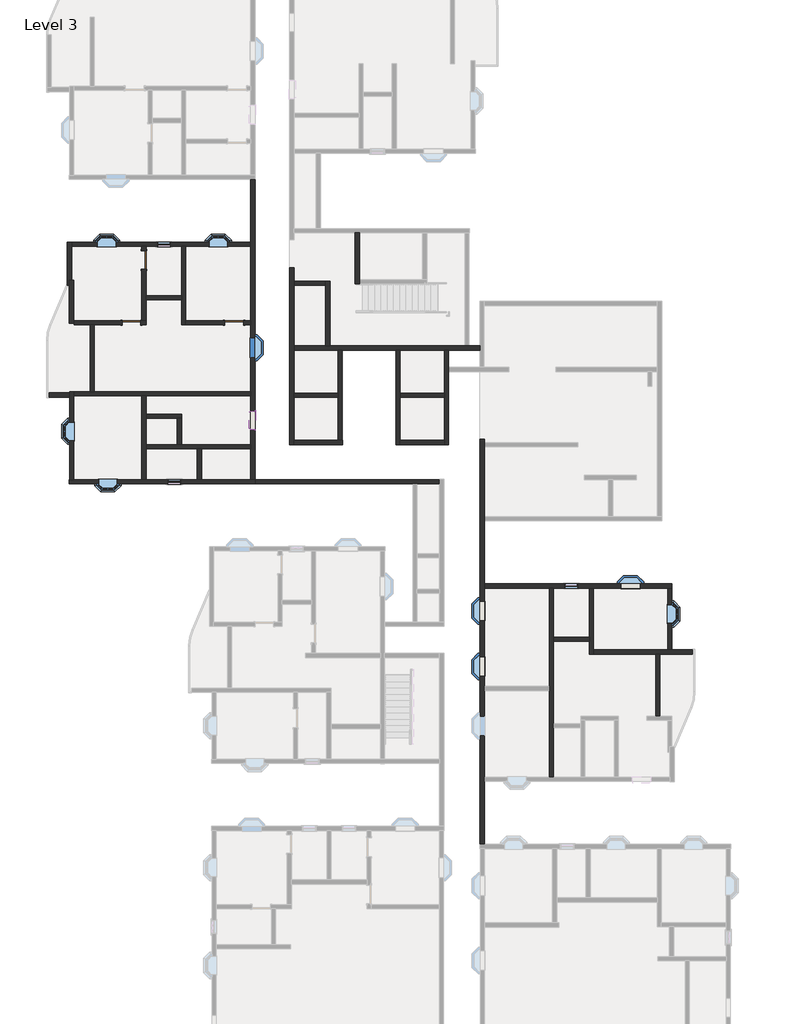
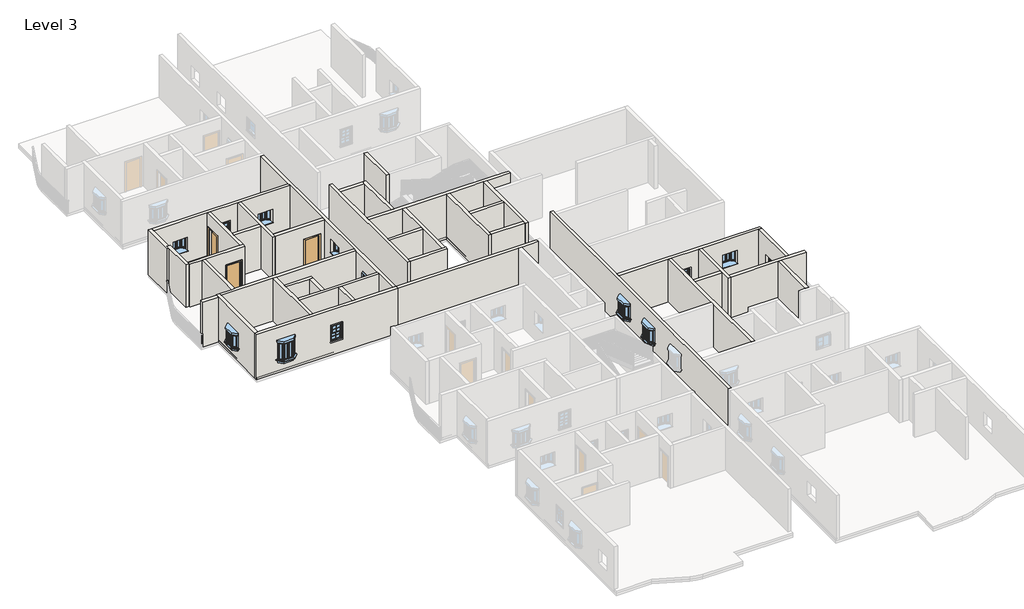
# One storey, part 3 of 14: 40 walls, 13 windows, 3 doors.
# Revit data of these elements (continued)
# Element 26 (IfcWall, "9\"")
#   Top Offset = 0' - 0"
#   Base Offset = 0' - 0"
#   wall height = 10' - 0"
#   Phase Created = New Construction
#   Base Constraint = Level 3
#   Top Constraint = Level 4
#   Materials on its faces: "Default Wall", "Earth"
# Element 27 (IfcWall, "9\"")
#   Top Offset = 0' - 0"
#   Base Offset = 0' - 0"
#   wall height = 10' - 0"
#   Phase Created = New Construction
#   Base Constraint = Level 3
#   Top Constraint = Level 4
#   Materials on its faces: "Default Wall", "Default Mass Interior Wall"
# Element 28 (IfcWall, "9\"")
#   Top Offset = 0' - 0"
#   Base Offset = 0' - 0"
#   wall height = 10' - 0"
#   Phase Created = New Construction
#   Base Constraint = Level 3
#   Top Constraint = Level 4
#   Materials on its faces: "Default Wall"
# Element 29 (IfcWall, "9\"")
#   Top Offset = 0' - 0"
#   Base Offset = 0' - 0"
#   wall height = 10' - 0"
#   Phase Created = New Construction
#   Base Constraint = Level 3
#   Top Constraint = Level 4
#   Materials on its faces: "Default Wall", "Default Mass Interior Wall", "Earth"
# Elements 30, 33, 34, 35, 36, 37, 38, 39, 40, 41 (IfcWall, "9\" w")
#   Top Offset = 0' - 0"
#   Base Offset = 0' - 0"
#   wall height = 10' - 0"
#   Phase Created = New Construction
#   Base Constraint = Level 3
#   Top Constraint = Level 4
#   Materials on its faces: "Default Wall"
# Element 31 (IfcWall, "9\" w")
#   Top Offset = 0' - 0"
#   Base Offset = 0' - 0"
#   wall height = 10' - 0"
#   Phase Created = New Construction
#   Base Constraint = Level 3
#   Top Constraint = Level 4
#   Materials on its faces: "Default Wall", "Earth"
# Element 32 (IfcWall, "9\" w")
#   Top Offset = 0' - 0"
#   Base Offset = 0' - 0"
#   wall height = 10' - 0"
#   Phase Created = New Construction
#   Base Constraint = Level 3
#   Top Constraint = Level 4
#   Materials on its faces: "Default Wall", "Brick, Soldier Course"
# Element 42 (IfcWall, "9\" w")
#   Top Offset = 0' - 0"
#   Base Offset = 0' - 0"
#   wall height = 10' - 0"
#   Phase Created = New Construction
#   Base Constraint = Level 3
#   Top Constraint = Level 4
#   Materials on its faces: "Default Wall", "Wood - Stained"
# Element 43 (IfcWall, "9\" w")
#   Top Offset = 0' - 0"
#   Base Offset = 0' - 0"
#   wall height = 10' - 0"
#   Phase Created = New Construction
#   Base Constraint = Level 3
#   Top Constraint = Level 4
#   Materials on its faces: "Default Wall", "Acoustic Ceiling Tile 24 x 24"
# Element 44 (IfcWindow, "910x1210mm")
#   Mark = "304"
#   Phase Created = New Construction
#   Materials on its faces: "Window Frame", "Glass"
# Element 45 (IfcWindow, "910x910mm")
#   Mark = "145"
#   Phase Created = New Construction
#   Materials on its faces: "Window Frame", "Glass"
# Element 46 (IfcWindow, "910x910mm")
#   Mark = "146"
#   Phase Created = New Construction
#   Materials on its faces: "Window Frame", "Glass"
# Element 47 (IfcWindow, "910x910mm")
#   Mark = "118"
#   Phase Created = New Construction
#   Materials on its faces: "Window Frame", "Glass"
# Element 48 (IfcWindow, "910x910mm")
#   Mark = "119"
#   Phase Created = New Construction
#   Materials on its faces: "Window Frame", "Glass"
# Element 49 (IfcWindow, "910x910mm")
#   Mark = "120"
#   Phase Created = New Construction
#   Materials on its faces: "Window Frame", "Glass"
# Element 50 (IfcWindow, "910x910mm")
#   Mark = "121"
#   Phase Created = New Construction
#   Materials on its faces: "Window Frame", "Glass"
# Element 51 (IfcWindow, "910x910mm")
#   Mark = "143"
#   Phase Created = New Construction
#   Materials on its faces: "Window Frame", "Glass"
# Element 52 (IfcWindow, "910x910mm")
#   Mark = "144"
#   Phase Created = New Construction
#   Materials on its faces: "Window Frame", "Glass"
# Element 53 (IfcWindow, "Window-Double-Hung : 26\" x 42\"")
#   Mark = "167"
#   Window Inset = 0' - 0"
#   Interior Wall Closure = 0' - 1 1/2"
#   Frame Extension = 0' - 1 1/4"
#   Exterior Wall Closure = 0' - 0 1/2"
#   Interior Trim Visibility = yes
#   Indicator Visibility = yes
#   Exterior Trim Visibility = yes
#   Phase Created = New Construction
#   Materials on its faces: "Wood - Stained", "Glass", "Clad - White"
# Element 54 (IfcWindow, "Window-Double-Hung : 26\" x 42\"")
#   Mark = "156"
#   Window Inset = 0' - 0"
#   Interior Wall Closure = 0' - 1 1/2"
#   Frame Extension = 0' - 1 1/4"
#   Exterior Wall Closure = 0' - 0 1/2"
#   Interior Trim Visibility = yes
#   Indicator Visibility = yes
#   Exterior Trim Visibility = yes
#   Phase Created = New Construction
#   Materials on its faces: "Wood - Stained", "Glass", "Clad - White"
# Element 55 (IfcWindow, "Window-Double-Hung : 26\" x 42\"")
#   Mark = "157"
#   Window Inset = 0' - 0"
#   Interior Wall Closure = 0' - 1 1/2"
#   Frame Extension = 0' - 1 1/4"
#   Exterior Wall Closure = 0' - 0 1/2"
#   Interior Trim Visibility = yes
#   Indicator Visibility = yes
#   Exterior Trim Visibility = yes
#   Phase Created = New Construction
#   Materials on its faces: "Wood - Stained", "Glass", "Clad - White"
# Element 56 (IfcWindow, "Windows_Sgl_w-Glazing_Bars : 910x910mm")
#   Mark = "152"
#   Phase Created = New Construction
#   Materials on its faces: "Window Frame", "Glass"
# Materials
#   "Door - Panel": class "Wood", colour RGB 210 159 95, transparency 0, Cost = 0
#   "Door - Frame": colour RGB 118 70 51, transparency 0, Cost = 0
#   "Window Frame": colour RGB 249 249 249, transparency 0
#   "Glass": class "Glass", colour RGB 0 128 192, transparency 0.75, Description = "Soda Lime Glass", Cost = 0
#   "Wood - Stained": class "Wood", colour RGB 224 178 126, transparency 0, Cost = 0
#   "Clad - White": class "Wood", colour RGB 242 242 238, transparency 0, Cost = 0
#   "Default Wall": colour RGB 128 128 128, transparency 0, Cost = 0
#   "Cherry": class "Wood", colour RGB 226 177 128, transparency 0, Description = "Prunus Serotina", Cost = 0
#   "Parking Stripe": class "Paint", colour RGB 250 250 91, transparency 0, Cost = 0
#   "Earth": class "Generic", colour RGB 97 75 62, transparency 0, Description = "Soil", Cost = 0
#   "Default Mass Interior Wall": class "Generic", colour RGB 195 229 126, transparency 0, Cost = 0
#   "Brick, Soldier Course": class "Masonry", colour RGB 170 98 104, transparency 0, Description = "Common brick soldier coursed", Cost = 0
#   "Acoustic Ceiling Tile 24 x 24": class "Generic", colour RGB 232 232 232, transparency 0, Description = "Acoustic Ceiling Tile 24 x 24", Cost = 0
